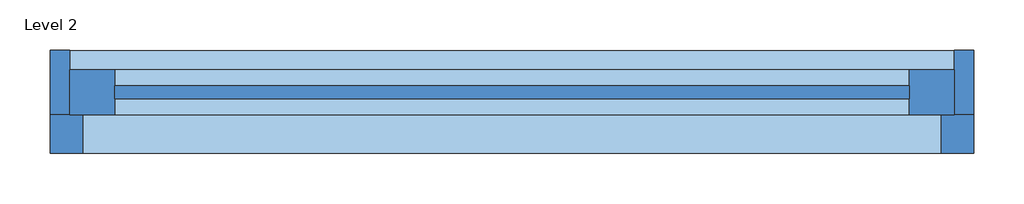
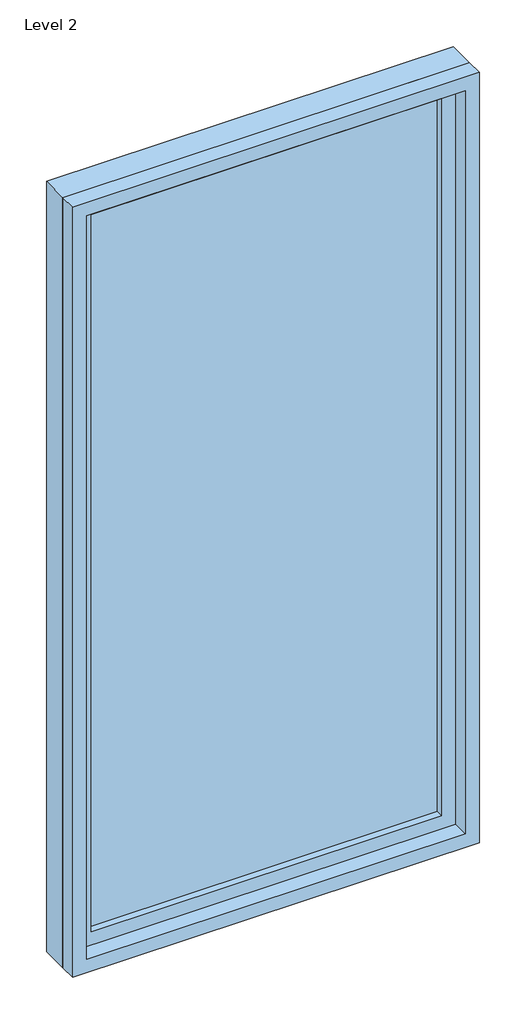
# One storey: 1 window.
"""IFC4 building model written with IfcOpenShell, lengths in millimetres."""

from ifc_helpers import new_model, si_unit, origin, place, context, project, spatial, transform, mapped, element, save
from components import window_8ce0b82f

model = new_model("IFC4")

# Units and contexts
model_context = context("Model", 3, world=origin())
ifc_project = project(units=[si_unit("LENGTHUNIT", "METRE", prefix="MILLI")], contexts=[model_context])

# Site, building, storey
site = spatial("IfcSite", under=ifc_project)
building = spatial("IfcBuilding", under=site)
storey = spatial("IfcBuildingStorey", under=building, Name="Level 2", Elevation=3048.0)

# Window
placement = place(None, origin())
window_shape = window_8ce0b82f(model_context)
element("IfcWindow", 1, ObjectType="Fixed : 36\" x 72\"", at=placement, inside=storey, context=model_context, shape_type="MappedRepresentation", body=[
    mapped(window_shape, transform((-7732.7069895, -8391.1980299, 3048.0), x_axis=(1.0, 0.0, 0.0), y_axis=(0.0, 1.0, 0.0), z_axis=(0.0, 0.0, 1.0))),
])

save(model, "model.ifc")

# Revit data of these elements
# Type "Fixed : 36\" x 72\""
#   Type Mark = "9"
#   Construction Type Id = "GSP4R"
#   Assembly Code = "B2020100"
#   Analytic Construction = "1/8 in Pilkington single glazing"
#   Visual Light Transmittance = 0.9
#   Solar Heat Gain Coefficient = 0.78
#   Heat Transfer Coefficient (U) = 0.6496 BTU/(h·ft²·°F)
#   Height = 6' - 0"
#   Default Sill Height = 1' - 0"
#   Width = 3' - 0"
#   Window Inset = 0' - 0 3/4"
#   Define Thermal Properties by = 1
#   Glass Pane Material = Glass
#   Sash Material = Sash
#   Wall Closure = (empty or 0)
# Element 1 (IfcWindow, "Fixed : 36\" x 72\"")
#   Mark = "2"
#   Phase Created = New Construction
#   Materials on its faces: "Sash", "Glass"
# Materials
#   "Glass": class "Glass", colour RGB 0 128 192, transparency 0.75, Description = "Soda Lime Glass", Cost = 0
#   "Sash": class "Wood", colour RGB 224 178 126, transparency 0
